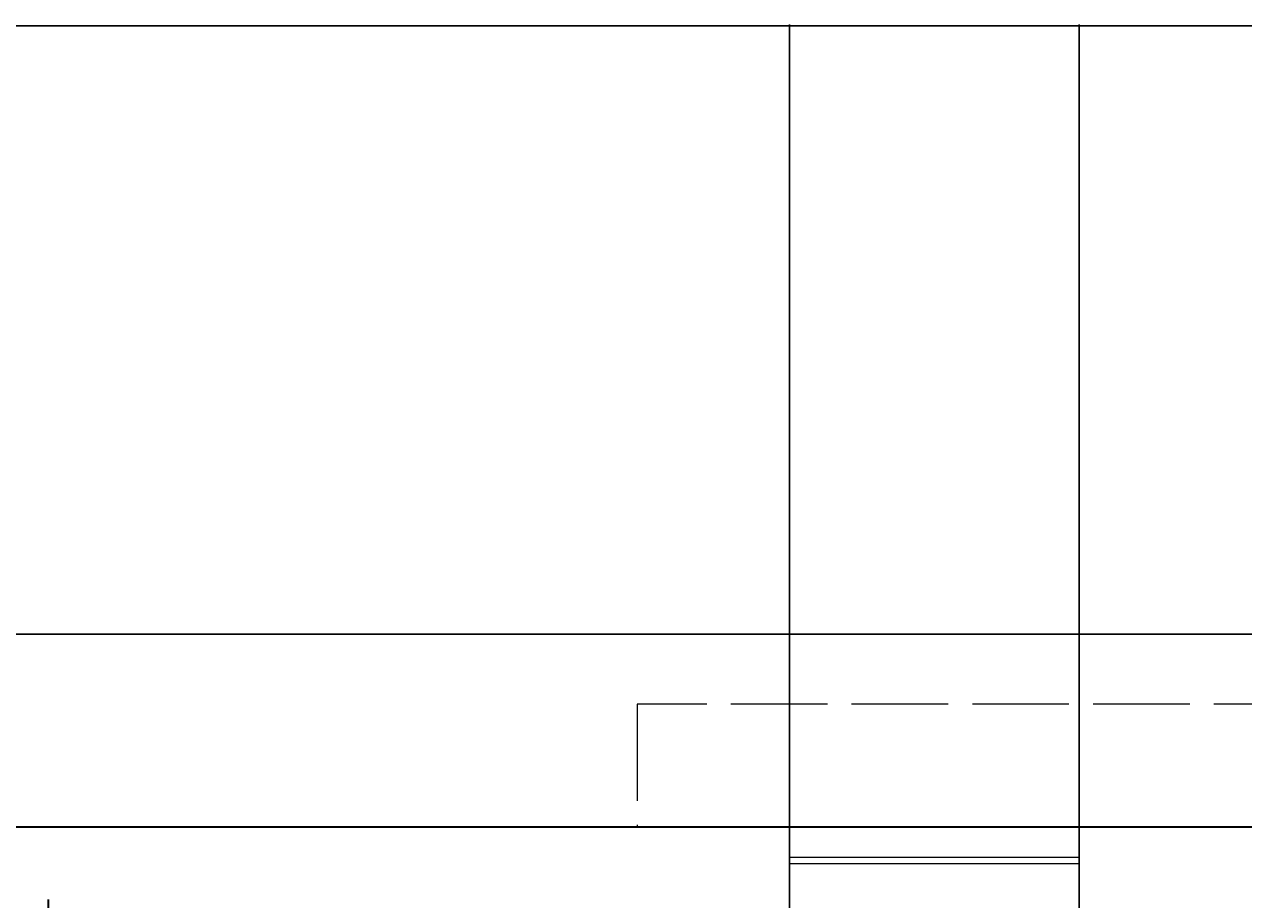
# Model space of a CAD drawing. Units: inches. Extents: x -61 to 1599, y -1316 to 257.
# Tile 124 of 204: x 85 to 236, y 149 to 257. Entities that reach past the tile are written whole.
import ezdxf

# ---------------------------------------------------------------- set-up
doc = ezdxf.new("R2010")
doc.units = ezdxf.units.IN
doc.header["$MEASUREMENT"] = 0
doc.linetypes.add('ACAD_ISO02W100', pattern=[15, 12, -3])
for name, color, linetype, lineweight in [('A-ANNO-DIMS', 2, 'Continuous', 18), ('A-FLOR-OVHD', 203, 'ACAD_ISO02W100', 13), ('WALLS', 4, 'Continuous', 35), ('WINDOWS', 220, 'Continuous', 18)]:
    doc.layers.add(name, color=color, linetype=linetype, lineweight=lineweight)
doc.styles.get("Standard").update_dxf_attribs({"font": 'arial.ttf'})
doc.dimstyles.get("Standard").update_dxf_attribs({"dimtxt": 0.18, "dimasz": 0.18, "dimexe": 0.18, "dimexo": 0.0625, "dimgap": 0.09, "dimtad": 0, "dimtih": 1, "dimtoh": 1, "dimdec": 0, "dimzin": 0, "dimdsep": 46, "dimlunit": 3, "dimtxsty": 'Standard', "dimcen": 0.09, "dimadec": 0, "dimazin": 0, "dimtfac": 1, "dimtdec": 0, "dimtofl": 0, "dimtmove": 0, "dimatfit": 3, "dimfxl": 1, "dimtolj": 1, "dimtzin": 0, "dimarcsym": 0})

# ---------------------------------------------------------------- blocks, each defined once
blk = doc.blocks.new('WIN-36IN')
for p, q in [((0, 4.5), (0, 9)), ((0, 9), (0, 0)), ((36, 9), (36, 0)), ((0, 5.26), (36, 5.26)), ((0, 4.5), (36, 4.5)), ((0, 4.5), (36, 4.5))]:
    blk.add_line(p, q)
blk = doc.blocks.new('*D686')
at = {"layer": 'A-ANNO-DIMS', "color": 0, "lineweight": -2, "transparency": 16777216}
for p, q in [((14.7, 157.74), (14.7, 257.46)), ((14.88, 257.28), (768.35, 257.28)), ((1522.52, 257.28), (769.05, 257.28)), ((1522.7, 157.74), (1522.7, 257.46))]:
    blk.add_line(p, q, dxfattribs=at)
at = {"layer": 'A-ANNO-DIMS', "color": 0, "transparency": 16777216}
for points in [[(14.88, 257.31), (14.88, 257.25), (14.7, 257.28)], [(1522.52, 257.31), (1522.52, 257.25), (1522.7, 257.28)]]:
    blk.add_solid(points, dxfattribs=at)
at = {"layer": 'DEFPOINTS', "color": 0, "transparency": 16777216}
for p in [(1522.7, 257.28), (14.7, 157.68), (1522.7, 157.68)]:
    blk.add_point(p, dxfattribs=at)
at = {"layer": 'A-ANNO-DIMS', "color": 0, "transparency": 16777216, "insert": (768.7, 257.28), "char_height": 0.18, "attachment_point": 5}
blk.add_mtext('\\A1;1508', dxfattribs=at)
blk = doc.blocks.new('*D687')
at = {"layer": 'A-ANNO-DIMS', "color": 0, "lineweight": -2, "transparency": 16777216}
for p, q in [((289.42, 181.68), (-61.08, 181.68)), ((-60.9, 181.5), (-60.9, -528.95)), ((-60.9, -1239.76), (-60.9, -529.32)), ((319.64, -1239.94), (-61.08, -1239.94))]:
    blk.add_line(p, q, dxfattribs=at)
at = {"layer": 'A-ANNO-DIMS', "color": 0, "transparency": 16777216}
for points in [[(-60.93, 181.5), (-60.87, 181.5), (-60.9, 181.68)], [(-60.93, -1239.76), (-60.87, -1239.76), (-60.9, -1239.94)]]:
    blk.add_solid(points, dxfattribs=at)
at = {"layer": 'DEFPOINTS', "color": 0, "transparency": 16777216}
for p in [(289.48, 181.68), (-60.9, -1239.94), (319.7, -1239.94)]:
    blk.add_point(p, dxfattribs=at)
at = {"layer": 'A-ANNO-DIMS', "color": 0, "transparency": 16777216, "insert": (-60.9, -529.13), "char_height": 0.18, "attachment_point": 5}
blk.add_mtext('\\A1;1421.6', dxfattribs=at)
blk = doc.blocks.new('*D700')
at = {"layer": 'A-ANNO-DIMS', "color": 0, "lineweight": -2, "transparency": 16777216}
for p, q in [((14.7, -616.88), (14.7, 257.46)), ((14.88, 257.28), (96.77, 257.28)), ((179.57, 257.28), (97.68, 257.28)), ((179.75, -616.88), (179.75, 257.46))]:
    blk.add_line(p, q, dxfattribs=at)
at = {"layer": 'A-ANNO-DIMS', "color": 0, "transparency": 16777216}
for points in [[(14.88, 257.31), (14.88, 257.25), (14.7, 257.28)], [(179.57, 257.31), (179.57, 257.25), (179.75, 257.28)]]:
    blk.add_solid(points, dxfattribs=at)
at = {"layer": 'DEFPOINTS', "color": 0, "transparency": 16777216}
for p in [(179.75, 257.28), (14.7, -616.94), (179.75, -616.94)]:
    blk.add_point(p, dxfattribs=at)
at = {"layer": 'A-ANNO-DIMS', "color": 0, "transparency": 16777216, "insert": (97.23, 257.28), "char_height": 0.18, "attachment_point": 5}
blk.add_mtext('\\A1;165.05', dxfattribs=at)
blk = doc.blocks.new('*D701')
at = {"layer": 'A-ANNO-DIMS', "color": 0, "lineweight": -2, "transparency": 16777216}
for p, q in [((215.75, -616.88), (215.75, 257.46)), ((215.93, 257.28), (233.92, 257.28)), ((252.7, 257.28), (234.71, 257.28)), ((252.88, -616.88), (252.88, 257.46))]:
    blk.add_line(p, q, dxfattribs=at)
at = {"layer": 'A-ANNO-DIMS', "color": 0, "transparency": 16777216}
for points in [[(215.93, 257.31), (215.93, 257.25), (215.75, 257.28)], [(252.7, 257.31), (252.7, 257.25), (252.88, 257.28)]]:
    blk.add_solid(points, dxfattribs=at)
at = {"layer": 'DEFPOINTS', "color": 0, "transparency": 16777216}
for p in [(252.88, 257.28), (215.75, -616.94), (252.88, -616.94)]:
    blk.add_point(p, dxfattribs=at)
at = {"layer": 'A-ANNO-DIMS', "color": 0, "transparency": 16777216, "insert": (234.32, 257.28), "char_height": 0.18, "attachment_point": 5}
blk.add_mtext('\\A1;37.13', dxfattribs=at)

msp = doc.modelspace()

# ---------------------------------------------------------------- linework, layer by layer
at = {"layer": 'A-FLOR-OVHD'}
for p, q in [((289.4807, 172.9695), (160.8585, 172.9695)), ((160.8585, 172.9695), (160.8585, 157.6771))]:
    msp.add_line(p, q, dxfattribs=at)
at = {"layer": 'WALLS'}
for p, q in [((544.7028, 157.6771), (14.7028, 157.6771)), ((87.7028, 148.6771), (87.7028, -7.3229))]:
    msp.add_line(p, q, dxfattribs=at)

# ---------------------------------------------------------------- block references
at = {"layer": 'WINDOWS'}
msp.add_blockref('WIN-36IN', (179.752, 148.677), dxfattribs=at)

# ---------------------------------------------------------------- dimensions: what is measured, and where the dimension line sits
at = {"layer": 'A-ANNO-DIMS'}
for base, p1, p2, override, picture, middle in [((1522.7028, 257.2771), (14.7028, 157.6771), (1522.7028, 157.6771), {"dimdec": 0, "dimlfac": 1, "dimrnd": 0, "dimzin": 0, "dimdsep": 46, "dimlunit": 2}, '*D686', (768.7028, 257.2771)), ((179.7521, 257.2771), (14.7028, -616.9446), (179.7521, -616.9446), {"dimdec": 2, "dimlfac": 1, "dimrnd": 0, "dimzin": 0, "dimdsep": 46, "dimlunit": 2}, '*D700', (97.2274, 257.2771)), ((252.8825, 257.2771), (215.7521, -616.9446), (252.8825, -616.9446), {"dimdec": 2, "dimlfac": 1, "dimrnd": 0, "dimzin": 0, "dimdsep": 46, "dimlunit": 2}, '*D701', (234.3173, 257.2771))]:
    dim = msp.add_linear_dim(base=base, p1=p1, p2=p2, dimstyle='Standard', override=override, dxfattribs=at)
    dim.commit()
    dim.dimension.update_dxf_attribs({"geometry": picture, "text_midpoint": middle})
dim = msp.add_linear_dim(base=(-60.8972, -1239.9446), p1=(289.4807, 181.6771), p2=(319.7028, -1239.9446), angle=90, dimstyle='Standard', override={"dimdec": 1, "dimlfac": 1, "dimrnd": 0, "dimzin": 0, "dimdsep": 46, "dimlunit": 2}, dxfattribs=at)
dim.commit()
dim.dimension.update_dxf_attribs({"geometry": '*D687', "text_midpoint": (-60.8972, -529.1337)})

doc.saveas('drawing.dxf')
